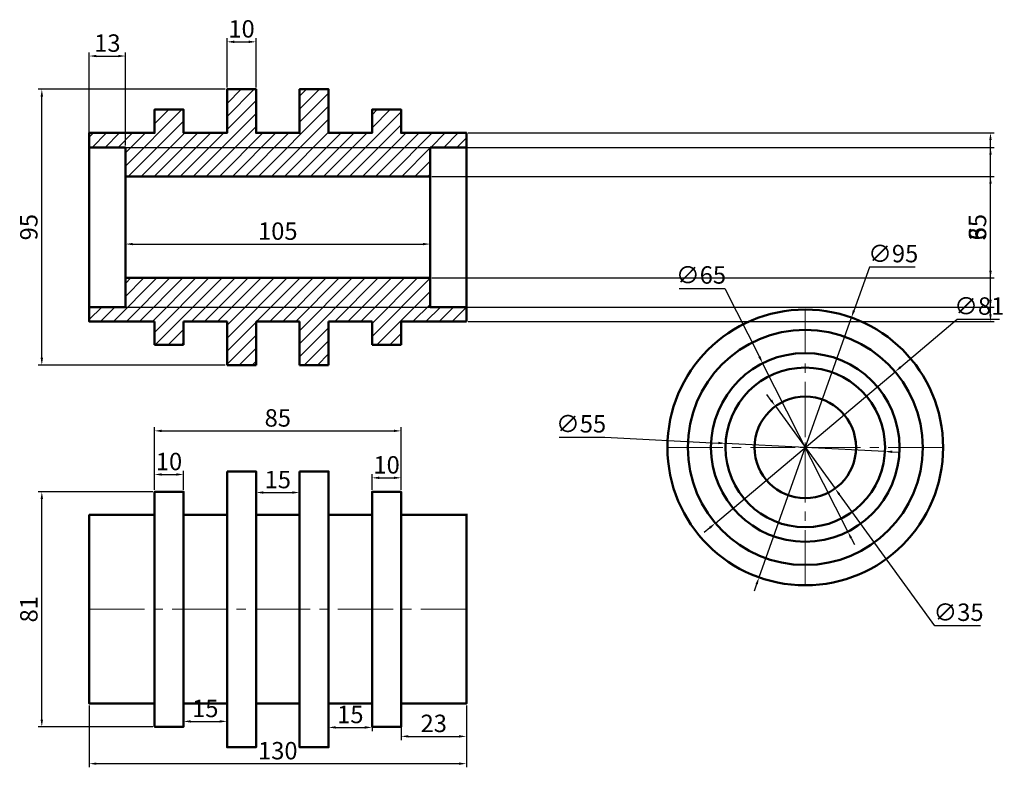
# Model space of a CAD drawing. Units: millimetres. Extents: x 106 to 445, y 110 to 368.
import ezdxf

# ---------------------------------------------------------------- set-up
doc = ezdxf.new("R2010")
doc.units = ezdxf.units.MM
doc.linetypes.add('CENTER2', pattern=[28.575, 19.05, -3.175, 3.175, -3.175])
for name, color, linetype, lineweight in [('M-CNTR', 4, 'CENTER2', 18), ('M-DIMS', 2, 'Continuous', 25), ('M-HATC', 8, 'Continuous', 18), ('M-OUTL', 7, 'Continuous', 50)]:
    doc.layers.add(name, color=color, linetype=linetype, lineweight=lineweight)
doc.styles.get("Standard").update_dxf_attribs({"font": 'arial.ttf'})
doc.dimstyles.new('ISO-25', dxfattribs={"dimtxt": 6, "dimasz": 2.5, "dimexe": 1.25, "dimexo": 0.625, "dimtad": 1, "dimtoh": 1, "dimdec": 0, "dimtxsty": 'Standard', "dimcen": 2.5, "dimadec": 0, "dimazin": 0, "dimtfac": 1, "dimtdec": 0, "dimtmove": 0, "dimatfit": 3, "dimfxl": 1, "dimarcsym": 0})

# ---------------------------------------------------------------- blocks, each defined once
blk = doc.blocks.new('*D1')
at = {"layer": 'Defpoints', "color": 0, "transparency": 16777216}
for p in [(142.24, 355.39), (129.74, 323.93), (142.24, 323.93)]:
    blk.add_point(p, dxfattribs=at)
at = {"layer": 'M-DIMS', "color": 0, "lineweight": -2, "transparency": 16777216}
for p, q in [((129.74, 324.56), (129.74, 356.64)), ((142.24, 324.56), (142.24, 356.64)), ((132.24, 355.39), (139.74, 355.39))]:
    blk.add_line(p, q, dxfattribs=at)
at = {"layer": 'M-DIMS', "color": 0, "transparency": 16777216}
for points in [[(132.24, 355.81), (132.24, 354.98), (129.74, 355.39)], [(139.74, 355.81), (139.74, 354.98), (142.24, 355.39)]]:
    blk.add_solid(points, dxfattribs=at)
at = {"layer": 'M-DIMS', "color": 0, "transparency": 16777216, "insert": (135.99, 359.08), "char_height": 6, "attachment_point": 5}
blk.add_mtext('13', dxfattribs=at)
blk = doc.blocks.new('*D2')
at = {"layer": 'Defpoints', "color": 0, "transparency": 16777216}
for p in [(142.24, 296.43), (247.24, 296.43), (247.24, 290.61)]:
    blk.add_point(p, dxfattribs=at)
at = {"layer": 'M-DIMS', "color": 0, "lineweight": -2, "transparency": 16777216}
for p, q in [((142.24, 295.81), (142.24, 289.36)), ((247.24, 295.81), (247.24, 289.36)), ((144.74, 290.61), (244.74, 290.61))]:
    blk.add_line(p, q, dxfattribs=at)
at = {"layer": 'M-DIMS', "color": 0, "transparency": 16777216}
for points in [[(144.74, 291.03), (144.74, 290.2), (142.24, 290.61)], [(244.74, 291.03), (244.74, 290.2), (247.24, 290.61)]]:
    blk.add_solid(points, dxfattribs=at)
at = {"layer": 'M-DIMS', "color": 0, "transparency": 16777216, "insert": (194.74, 294.3), "char_height": 6, "attachment_point": 5}
blk.add_mtext('105', dxfattribs=at)
blk = doc.blocks.new('*D3')
at = {"layer": 'Defpoints', "color": 0, "transparency": 16777216}
for p in [(237.24, 226.26), (152.24, 205.31), (237.24, 205.31)]:
    blk.add_point(p, dxfattribs=at)
at = {"layer": 'M-DIMS', "color": 0, "lineweight": -2, "transparency": 16777216}
for p, q in [((152.24, 205.93), (152.24, 227.51)), ((237.24, 205.93), (237.24, 227.51)), ((154.74, 226.26), (234.74, 226.26))]:
    blk.add_line(p, q, dxfattribs=at)
at = {"layer": 'M-DIMS', "color": 0, "transparency": 16777216}
for points in [[(154.74, 226.68), (154.74, 225.84), (152.24, 226.26)], [(234.74, 226.68), (234.74, 225.84), (237.24, 226.26)]]:
    blk.add_solid(points, dxfattribs=at)
at = {"layer": 'M-DIMS', "color": 0, "transparency": 16777216, "insert": (194.74, 229.95), "char_height": 6, "attachment_point": 5}
blk.add_mtext('85', dxfattribs=at)
blk = doc.blocks.new('*D4')
at = {"layer": 'Defpoints', "color": 0, "transparency": 16777216}
for p in [(129.74, 132.31), (259.74, 132.31), (259.74, 111.62)]:
    blk.add_point(p, dxfattribs=at)
at = {"layer": 'M-DIMS', "color": 0, "lineweight": -2, "transparency": 16777216}
for p, q in [((129.74, 131.68), (129.74, 110.37)), ((259.74, 131.68), (259.74, 110.37)), ((132.24, 111.62), (257.24, 111.62))]:
    blk.add_line(p, q, dxfattribs=at)
at = {"layer": 'M-DIMS', "color": 0, "transparency": 16777216}
for points in [[(132.24, 112.03), (132.24, 111.2), (129.74, 111.62)], [(257.24, 112.03), (257.24, 111.2), (259.74, 111.62)]]:
    blk.add_solid(points, dxfattribs=at)
at = {"layer": 'M-DIMS', "color": 0, "transparency": 16777216, "insert": (194.74, 115.31), "char_height": 6, "attachment_point": 5}
blk.add_mtext('130', dxfattribs=at)
blk = doc.blocks.new('*D5')
at = {"layer": 'Defpoints', "color": 0, "transparency": 16777216}
for p in [(162.24, 132.3), (177.24, 132.3), (177.24, 126.18)]:
    blk.add_point(p, dxfattribs=at)
at = {"layer": 'M-DIMS', "color": 0, "lineweight": -2, "transparency": 16777216}
for p, q in [((162.24, 131.67), (162.24, 124.93)), ((177.24, 131.67), (177.24, 124.93)), ((164.74, 126.18), (174.74, 126.18))]:
    blk.add_line(p, q, dxfattribs=at)
at = {"layer": 'M-DIMS', "color": 0, "transparency": 16777216}
for points in [[(164.74, 126.6), (164.74, 125.76), (162.24, 126.18)], [(174.74, 126.6), (174.74, 125.76), (177.24, 126.18)]]:
    blk.add_solid(points, dxfattribs=at)
at = {"layer": 'M-DIMS', "color": 0, "transparency": 16777216, "insert": (169.74, 129.87), "char_height": 6, "attachment_point": 5}
blk.add_mtext('15', dxfattribs=at)
blk = doc.blocks.new('*D6')
at = {"layer": 'Defpoints', "color": 0, "transparency": 16777216}
for p in [(162.24, 211.24), (152.24, 205.31), (162.24, 205.31)]:
    blk.add_point(p, dxfattribs=at)
at = {"layer": 'M-DIMS', "color": 0, "lineweight": -2, "transparency": 16777216}
for p, q in [((152.24, 205.93), (152.24, 212.49)), ((154.74, 211.24), (159.74, 211.24)), ((162.24, 205.93), (162.24, 212.49))]:
    blk.add_line(p, q, dxfattribs=at)
at = {"layer": 'M-DIMS', "color": 0, "transparency": 16777216}
for points in [[(154.74, 211.66), (154.74, 210.83), (152.24, 211.24)], [(159.74, 211.66), (159.74, 210.83), (162.24, 211.24)]]:
    blk.add_solid(points, dxfattribs=at)
at = {"layer": 'M-DIMS', "color": 0, "transparency": 16777216, "insert": (157.24, 214.93), "char_height": 6, "attachment_point": 5}
blk.add_mtext('10', dxfattribs=at)
blk = doc.blocks.new('*D7')
at = {"layer": 'Defpoints', "color": 0, "transparency": 16777216}
for p in [(237.24, 210.09), (227.24, 205.3), (237.24, 205.31)]:
    blk.add_point(p, dxfattribs=at)
at = {"layer": 'M-DIMS', "color": 0, "lineweight": -2, "transparency": 16777216}
for p, q in [((227.24, 205.92), (227.24, 211.34)), ((237.24, 205.93), (237.24, 211.34)), ((229.74, 210.09), (234.74, 210.09))]:
    blk.add_line(p, q, dxfattribs=at)
at = {"layer": 'M-DIMS', "color": 0, "transparency": 16777216}
for points in [[(229.74, 210.51), (229.74, 209.67), (227.24, 210.09)], [(234.74, 210.51), (234.74, 209.67), (237.24, 210.09)]]:
    blk.add_solid(points, dxfattribs=at)
at = {"layer": 'M-DIMS', "color": 0, "transparency": 16777216, "insert": (232.24, 213.78), "char_height": 6, "attachment_point": 5}
blk.add_mtext('10', dxfattribs=at)
blk = doc.blocks.new('*D8')
at = {"layer": 'Defpoints', "color": 0, "transparency": 16777216}
for p in [(202.24, 205.02), (187.24, 197.31), (202.24, 197.31)]:
    blk.add_point(p, dxfattribs=at)
at = {"layer": 'M-DIMS', "color": 0, "lineweight": -2, "transparency": 16777216}
for p, q in [((187.24, 197.93), (187.24, 206.27)), ((189.74, 205.02), (199.74, 205.02)), ((202.24, 197.93), (202.24, 206.27))]:
    blk.add_line(p, q, dxfattribs=at)
at = {"layer": 'M-DIMS', "color": 0, "transparency": 16777216}
for points in [[(189.74, 205.44), (189.74, 204.61), (187.24, 205.02)], [(199.74, 205.44), (199.74, 204.61), (202.24, 205.02)]]:
    blk.add_solid(points, dxfattribs=at)
at = {"layer": 'M-DIMS', "color": 0, "transparency": 16777216, "insert": (194.74, 208.71), "char_height": 6, "attachment_point": 5}
blk.add_mtext('15', dxfattribs=at)
blk = doc.blocks.new('*D9')
at = {"layer": 'Defpoints', "color": 0, "transparency": 16777216}
for p in [(212.24, 132.3), (227.24, 132.3), (227.24, 124.11)]:
    blk.add_point(p, dxfattribs=at)
at = {"layer": 'M-DIMS', "color": 0, "lineweight": -2, "transparency": 16777216}
for p, q in [((212.24, 131.67), (212.24, 122.86)), ((227.24, 131.67), (227.24, 122.86)), ((214.74, 124.11), (224.74, 124.11))]:
    blk.add_line(p, q, dxfattribs=at)
at = {"layer": 'M-DIMS', "color": 0, "transparency": 16777216}
for points in [[(214.74, 124.52), (214.74, 123.69), (212.24, 124.11)], [(224.74, 124.52), (224.74, 123.69), (227.24, 124.11)]]:
    blk.add_solid(points, dxfattribs=at)
at = {"layer": 'M-DIMS', "color": 0, "transparency": 16777216, "insert": (219.74, 127.79), "char_height": 6, "attachment_point": 5}
blk.add_mtext('15', dxfattribs=at)
blk = doc.blocks.new('*D10')
at = {"layer": 'Defpoints', "color": 0, "transparency": 16777216}
for p in [(237.24, 132.3), (259.74, 132.3), (259.74, 121.02)]:
    blk.add_point(p, dxfattribs=at)
at = {"layer": 'M-DIMS', "color": 0, "lineweight": -2, "transparency": 16777216}
for p, q in [((237.24, 131.67), (237.24, 119.77)), ((259.74, 131.67), (259.74, 119.77)), ((239.74, 121.02), (257.24, 121.02))]:
    blk.add_line(p, q, dxfattribs=at)
at = {"layer": 'M-DIMS', "color": 0, "transparency": 16777216}
for points in [[(239.74, 121.44), (239.74, 120.61), (237.24, 121.02)], [(257.24, 121.44), (257.24, 120.61), (259.74, 121.02)]]:
    blk.add_solid(points, dxfattribs=at)
at = {"layer": 'M-DIMS', "color": 0, "transparency": 16777216, "insert": (248.49, 124.72), "char_height": 6, "attachment_point": 5}
blk.add_mtext('23', dxfattribs=at)
blk = doc.blocks.new('*D11')
at = {"layer": 'Defpoints', "color": 0, "transparency": 16777216}
for p in [(366.27, 234.72), (386.85, 206.41)]:
    blk.add_point(p, dxfattribs=at)
at = {"layer": 'M-DIMS', "color": 0, "lineweight": -2, "transparency": 16777216}
for p, q in [((364.8, 236.74), (363.33, 238.76)), ((366.27, 234.72), (386.85, 206.41)), ((421.18, 159.15), (388.32, 204.38)), ((436.98, 159.15), (421.18, 159.15))]:
    blk.add_line(p, q, dxfattribs=at)
at = {"layer": 'M-DIMS', "color": 0, "transparency": 16777216}
for points in [[(365.14, 236.99), (364.47, 236.5), (366.27, 234.72)], [(388.65, 204.63), (387.98, 204.14), (386.85, 206.41)]]:
    blk.add_solid(points, dxfattribs=at)
at = {"layer": 'M-DIMS', "color": 0, "transparency": 16777216, "insert": (429.39, 163.01), "char_height": 6, "attachment_point": 5}
blk.add_mtext('∅35', dxfattribs=at)
blk = doc.blocks.new('*D12')
at = {"layer": 'Defpoints', "color": 0, "transparency": 16777216}
for p in [(349.1, 221.96), (404.02, 219.17)]:
    blk.add_point(p, dxfattribs=at)
at = {"layer": 'M-DIMS', "color": 0, "lineweight": -2, "transparency": 16777216}
for p, q in [((291.71, 224.06), (307.5, 224.06)), ((307.5, 224.06), (346.6, 222.08)), ((404.02, 219.17), (349.1, 221.96)), ((406.52, 219.04), (409.02, 218.92))]:
    blk.add_line(p, q, dxfattribs=at)
at = {"layer": 'M-DIMS', "color": 0, "transparency": 16777216}
for points in [[(346.62, 222.5), (346.58, 221.67), (349.1, 221.96)], [(406.54, 219.46), (406.5, 218.63), (404.02, 219.17)]]:
    blk.add_solid(points, dxfattribs=at)
at = {"layer": 'M-DIMS', "color": 0, "transparency": 16777216, "insert": (299.29, 227.92), "char_height": 6, "attachment_point": 5}
blk.add_mtext('∅55', dxfattribs=at)
blk = doc.blocks.new('*D13')
at = {"layer": 'Defpoints', "color": 0, "transparency": 16777216}
for p in [(361.88, 249.56), (391.24, 191.57)]:
    blk.add_point(p, dxfattribs=at)
at = {"layer": 'M-DIMS', "color": 0, "lineweight": -2, "transparency": 16777216}
for p, q in [((333.05, 275.33), (348.84, 275.33)), ((348.84, 275.33), (360.75, 251.79)), ((391.24, 191.57), (361.88, 249.56)), ((392.37, 189.33), (393.5, 187.1))]:
    blk.add_line(p, q, dxfattribs=at)
at = {"layer": 'M-DIMS', "color": 0, "transparency": 16777216}
for points in [[(361.13, 251.98), (360.38, 251.6), (361.88, 249.56)], [(392.74, 189.52), (391.99, 189.15), (391.24, 191.57)]]:
    blk.add_solid(points, dxfattribs=at)
at = {"layer": 'M-DIMS', "color": 0, "transparency": 16777216, "insert": (340.63, 279.19), "char_height": 6, "attachment_point": 5}
blk.add_mtext('∅65', dxfattribs=at)
blk = doc.blocks.new('*D14')
at = {"layer": 'Defpoints', "color": 0, "transparency": 16777216}
for p in [(407.55, 246.64), (345.57, 194.49)]:
    blk.add_point(p, dxfattribs=at)
at = {"layer": 'M-DIMS', "color": 0, "lineweight": -2, "transparency": 16777216}
for p, q in [((428.93, 264.63), (409.46, 248.25)), ((443.52, 264.63), (428.93, 264.63)), ((345.57, 194.49), (407.55, 246.64)), ((343.66, 192.88), (341.75, 191.27))]:
    blk.add_line(p, q, dxfattribs=at)
at = {"layer": 'M-DIMS', "color": 0, "transparency": 16777216}
for points in [[(409.19, 248.57), (409.73, 247.93), (407.55, 246.64)], [(343.39, 193.2), (343.93, 192.56), (345.57, 194.49)]]:
    blk.add_solid(points, dxfattribs=at)
at = {"layer": 'M-DIMS', "color": 0, "transparency": 16777216, "insert": (436.54, 268.49), "char_height": 6, "attachment_point": 5}
blk.add_mtext('∅81', dxfattribs=at)
blk = doc.blocks.new('*D15')
at = {"layer": 'Defpoints', "color": 0, "transparency": 16777216}
for p in [(392.48, 265.31), (360.64, 175.81)]:
    blk.add_point(p, dxfattribs=at)
at = {"layer": 'M-DIMS', "color": 0, "lineweight": -2, "transparency": 16777216}
for p, q in [((398.67, 282.71), (393.32, 267.67)), ((414.46, 282.71), (398.67, 282.71)), ((360.64, 175.81), (392.48, 265.31)), ((359.8, 173.45), (358.96, 171.1))]:
    blk.add_line(p, q, dxfattribs=at)
at = {"layer": 'M-DIMS', "color": 0, "transparency": 16777216}
for points in [[(392.93, 267.81), (393.71, 267.53), (392.48, 265.31)], [(359.41, 173.59), (360.19, 173.32), (360.64, 175.81)]]:
    blk.add_solid(points, dxfattribs=at)
at = {"layer": 'M-DIMS', "color": 0, "transparency": 16777216, "insert": (406.88, 286.56), "char_height": 6, "attachment_point": 5}
blk.add_mtext('∅95', dxfattribs=at)
blk = doc.blocks.new('*D16')
at = {"layer": 'Defpoints', "color": 0, "transparency": 16777216}
for p in [(113.39, 343.93), (177.24, 343.93), (177.24, 248.93)]:
    blk.add_point(p, dxfattribs=at)
at = {"layer": 'M-DIMS', "color": 0, "lineweight": -2, "transparency": 16777216}
for p, q in [((176.62, 343.93), (112.14, 343.93)), ((113.39, 251.43), (113.39, 341.43)), ((176.62, 248.93), (112.14, 248.93))]:
    blk.add_line(p, q, dxfattribs=at)
at = {"layer": 'M-DIMS', "color": 0, "transparency": 16777216}
for points in [[(112.98, 341.43), (113.81, 341.43), (113.39, 343.93)], [(112.98, 251.43), (113.81, 251.43), (113.39, 248.93)]]:
    blk.add_solid(points, dxfattribs=at)
at = {"layer": 'M-DIMS', "color": 0, "transparency": 16777216, "insert": (109.7, 296.43), "char_height": 6, "attachment_point": 5, "rotation": 90}
blk.add_mtext('95', dxfattribs=at)
blk = doc.blocks.new('*D17')
at = {"layer": 'Defpoints', "color": 0, "transparency": 16777216}
for p in [(259.74, 328.93), (440.41, 328.93), (259.74, 263.93)]:
    blk.add_point(p, dxfattribs=at)
at = {"layer": 'M-DIMS', "color": 0, "lineweight": -2, "transparency": 16777216}
for p, q in [((260.37, 328.93), (441.66, 328.93)), ((440.41, 266.43), (440.41, 326.43)), ((260.37, 263.93), (441.66, 263.93))]:
    blk.add_line(p, q, dxfattribs=at)
at = {"layer": 'M-DIMS', "color": 0, "transparency": 16777216}
for points in [[(439.99, 326.43), (440.83, 326.43), (440.41, 328.93)], [(439.99, 266.43), (440.83, 266.43), (440.41, 263.93)]]:
    blk.add_solid(points, dxfattribs=at)
at = {"layer": 'M-DIMS', "color": 0, "transparency": 16777216, "insert": (436.72, 296.43), "char_height": 6, "attachment_point": 5, "rotation": 90}
blk.add_mtext('65', dxfattribs=at)
blk = doc.blocks.new('*D18')
at = {"layer": 'Defpoints', "color": 0, "transparency": 16777216}
for p in [(113.39, 205.31), (152.24, 205.31), (152.24, 124.31)]:
    blk.add_point(p, dxfattribs=at)
at = {"layer": 'M-DIMS', "color": 0, "lineweight": -2, "transparency": 16777216}
for p, q in [((151.62, 205.31), (112.14, 205.31)), ((113.39, 126.81), (113.39, 202.81)), ((151.62, 124.31), (112.14, 124.31))]:
    blk.add_line(p, q, dxfattribs=at)
at = {"layer": 'M-DIMS', "color": 0, "transparency": 16777216}
for points in [[(112.98, 202.81), (113.81, 202.81), (113.39, 205.31)], [(112.98, 126.81), (113.81, 126.81), (113.39, 124.31)]]:
    blk.add_solid(points, dxfattribs=at)
at = {"layer": 'M-DIMS', "color": 0, "transparency": 16777216, "insert": (109.7, 164.81), "char_height": 6, "attachment_point": 5, "rotation": 90}
blk.add_mtext('81', dxfattribs=at)
blk = doc.blocks.new('*D19')
at = {"layer": 'Defpoints', "color": 0, "transparency": 16777216}
for p in [(129.74, 323.93), (440.41, 323.93), (129.74, 268.93)]:
    blk.add_point(p, dxfattribs=at)
at = {"layer": 'M-DIMS', "color": 0, "lineweight": -2, "transparency": 16777216}
for p, q in [((130.37, 323.93), (441.66, 323.93)), ((440.41, 271.43), (440.41, 321.43)), ((130.37, 268.93), (441.66, 268.93))]:
    blk.add_line(p, q, dxfattribs=at)
at = {"layer": 'M-DIMS', "color": 0, "transparency": 16777216}
for points in [[(439.99, 321.43), (440.83, 321.43), (440.41, 323.93)], [(439.99, 271.43), (440.83, 271.43), (440.41, 268.93)]]:
    blk.add_solid(points, dxfattribs=at)
at = {"layer": 'M-DIMS', "color": 0, "transparency": 16777216, "insert": (436.73, 296.43), "char_height": 6, "attachment_point": 5, "rotation": 90}
blk.add_mtext('55', dxfattribs=at)
blk = doc.blocks.new('*D20')
at = {"layer": 'Defpoints', "color": 0, "transparency": 16777216}
for p in [(247.24, 313.93), (440.41, 313.93), (247.24, 278.93)]:
    blk.add_point(p, dxfattribs=at)
at = {"layer": 'M-DIMS', "color": 0, "lineweight": -2, "transparency": 16777216}
for p, q in [((247.87, 313.93), (441.66, 313.93)), ((440.41, 281.43), (440.41, 311.43)), ((247.87, 278.93), (441.66, 278.93))]:
    blk.add_line(p, q, dxfattribs=at)
at = {"layer": 'M-DIMS', "color": 0, "transparency": 16777216}
for points in [[(439.99, 311.43), (440.83, 311.43), (440.41, 313.93)], [(439.99, 281.43), (440.83, 281.43), (440.41, 278.93)]]:
    blk.add_solid(points, dxfattribs=at)
at = {"layer": 'M-DIMS', "color": 0, "transparency": 16777216, "insert": (436.72, 296.43), "char_height": 6, "attachment_point": 5, "rotation": 90}
blk.add_mtext('35', dxfattribs=at)
blk = doc.blocks.new('*D21')
at = {"layer": 'Defpoints', "color": 0, "transparency": 16777216}
for p in [(187.24, 360.28), (177.24, 343.93), (187.24, 343.93)]:
    blk.add_point(p, dxfattribs=at)
at = {"layer": 'M-DIMS', "color": 0, "lineweight": -2, "transparency": 16777216}
for p, q in [((177.24, 344.56), (177.24, 361.53)), ((179.74, 360.28), (184.74, 360.28)), ((187.24, 344.56), (187.24, 361.53))]:
    blk.add_line(p, q, dxfattribs=at)
at = {"layer": 'M-DIMS', "color": 0, "transparency": 16777216}
for points in [[(179.74, 360.7), (179.74, 359.87), (177.24, 360.28)], [(184.74, 360.7), (184.74, 359.87), (187.24, 360.28)]]:
    blk.add_solid(points, dxfattribs=at)
at = {"layer": 'M-DIMS', "color": 0, "transparency": 16777216, "insert": (182.24, 363.97), "char_height": 6, "attachment_point": 5}
blk.add_mtext('10', dxfattribs=at)

msp = doc.modelspace()

# ---------------------------------------------------------------- hatches: boundary and pattern name
at = {"layer": 'M-HATC'}
h = msp.add_hatch(dxfattribs=at)
h.set_pattern_fill('ANSI31', color=256)
h.set_pattern_definition([(45, (101.0912, 253.9006), (-2.245064, 2.245064), [])])
h.paths.add_polyline_path([(152.24, 328.93), (142.24, 328.93), (129.74, 328.93), (129.74, 323.93), (142.24, 323.93), (142.24, 313.93), (247.24, 313.93), (247.24, 323.93), (259.74, 323.93), (259.74, 328.93), (237.24, 328.93), (237.24, 336.93), (227.24, 336.93), (227.24, 328.93), (212.24, 328.93), (212.24, 343.93), (202.24, 343.93), (202.24, 328.93), (187.24, 328.93), (187.24, 343.93), (177.24, 343.93), (177.24, 328.93), (162.24, 328.93), (162.24, 336.93), (152.24, 336.93)])
h.paths.add_polyline_path([(142.24, 278.93), (142.24, 268.93), (129.74, 268.93), (129.74, 266.43), (129.74, 263.93), (142.24, 263.93), (152.24, 263.93), (152.24, 255.93), (162.24, 255.93), (162.24, 263.93), (177.24, 263.93), (177.24, 248.93), (187.24, 248.93), (187.24, 263.93), (202.24, 263.93), (202.24, 248.93), (212.24, 248.93), (212.24, 263.93), (227.24, 263.93), (227.24, 255.93), (237.24, 255.93), (237.24, 263.93), (259.74, 263.93), (259.74, 268.93), (247.24, 268.93), (247.24, 278.93)])

# ---------------------------------------------------------------- linework, layer by layer
at = {"layer": 'M-CNTR'}
for p, q in [((376.56, 224.06), (376.56, 268.06)), ((376.56, 218.81), (376.56, 222.31)), ((329.06, 220.56), (373.06, 220.56)), ((374.81, 220.56), (378.31, 220.56)), ((129.74, 164.81), (259.74, 164.81))]:
    msp.add_line(p, q, dxfattribs=at)
msp.add_lwpolyline([(376.56, 173.06), (376.56, 220.56), (424.06, 220.56)], dxfattribs=at)
at = {"layer": 'M-OUTL'}
for p, q in [((142.24, 313.93), (247.24, 313.93)), ((142.24, 278.93), (247.24, 278.93)), ((259.74, 268.93), (259.74, 263.93)), ((142.24, 263.93), (152.24, 263.93)), ((142.24, 263.93), (152.24, 263.93)), ((152.24, 263.93), (152.24, 255.93)), ((162.24, 255.93), (162.24, 263.93)), ((162.24, 263.93), (177.24, 263.93)), ((177.24, 263.93), (177.24, 248.93)), ((187.24, 248.93), (187.24, 263.93)), ((187.24, 263.93), (202.24, 263.93)), ((202.24, 263.93), (202.24, 248.93)), ((212.24, 248.93), (212.24, 263.93)), ((212.24, 263.93), (227.24, 263.93)), ((227.24, 263.93), (227.24, 255.93)), ((259.74, 263.93), (237.24, 263.93)), ((237.24, 255.93), (237.24, 263.93)), ((152.24, 255.93), (162.24, 255.93)), ((227.24, 255.93), (237.24, 255.93)), ((177.24, 248.93), (187.24, 248.93)), ((202.24, 248.93), (212.24, 248.93)), ((162.24, 197.31), (177.24, 197.31)), ((187.24, 197.31), (202.24, 197.31)), ((212.24, 197.31), (227.24, 197.31)), ((237.24, 197.31), (259.74, 197.31)), ((162.24, 132.3), (177.24, 132.3)), ((187.24, 132.3), (202.24, 132.3)), ((212.24, 132.3), (227.24, 132.3))]:
    msp.add_line(p, q, dxfattribs=at)
for points in [[(129.74, 323.93), (129.74, 328.93), (142.24, 328.93), (152.24, 328.93), (152.24, 336.93), (162.24, 336.93), (162.24, 328.93), (177.24, 328.93), (177.24, 343.93), (187.24, 343.93), (187.24, 328.93), (202.24, 328.93), (202.24, 343.93), (212.24, 343.93), (212.24, 328.93), (227.24, 328.93), (227.24, 336.93), (237.24, 336.93), (237.24, 328.93), (259.74, 328.93), (259.74, 323.93)], [(142.24, 263.93), (129.74, 263.93), (129.74, 268.93), (142.24, 268.93), (142.24, 323.93), (129.74, 323.93), (129.74, 266.43)], [(152.24, 197.31), (129.74, 197.31), (129.74, 132.31), (152.24, 132.31)], [(237.24, 132.3), (259.74, 132.3), (259.74, 197.74)]]:
    msp.add_lwpolyline(points, dxfattribs=at)
for points in [[(247.24, 323.93), (247.24, 268.93), (259.74, 268.93), (259.74, 323.93)], [(177.24, 212.31), (187.24, 212.31), (187.24, 117.3), (177.24, 117.3), (177.24, 197.56)], [(202.24, 212.31), (212.24, 212.31), (212.24, 117.3), (202.24, 117.3), (202.24, 197.74)], [(152.24, 197.31), (152.24, 205.31), (162.24, 205.31), (162.24, 124.31), (152.24, 124.31), (152.24, 132.31), (152.24, 164.81)], [(227.24, 124.3), (237.24, 124.3), (237.24, 205.3), (227.24, 205.3), (227.24, 197.74), (227.24, 132.3)]]:
    msp.add_lwpolyline(points, close=True, dxfattribs=at)
for radius in [47.5, 40.5, 32.5, 27.5, 17.5]:
    msp.add_circle((376.56, 220.56), radius, dxfattribs=at)

# ---------------------------------------------------------------- dimensions: what is measured, and where the dimension line sits
at = {"layer": 'M-DIMS'}
for base, p1, p2, override, picture, middle in [((187.24, 360.28), (177.24, 343.93), (187.24, 343.93), {"dimdec": 0, "dimlfac": 1, "dimrnd": 0, "dimzin": 0, "dimdsep": 46, "dimlunit": 2}, '*D21', (182.24, 363.97)), ((142.24278027, 355.39239272), (129.74278027, 323.93260068), (142.24278027, 323.93260068), {"dimclrd": 0, "dimclre": 0, "dimclrt": 0}, '*D1', (135.99278027, 359.08287703)), ((247.24, 290.61), (142.24, 296.43), (247.24, 296.43), {"dimclrd": 0, "dimclre": 0, "dimclrt": 0}, '*D2', (194.74, 294.3)), ((237.24, 226.26), (152.24, 205.31), (237.24, 205.31), {"dimclrd": 0, "dimclre": 0, "dimclrt": 0}, '*D3', (194.74, 229.95)), ((162.24, 211.24), (152.24, 205.31), (162.24, 205.31), {"dimclrd": 0, "dimclre": 0, "dimclrt": 0}, '*D6', (157.24, 214.93)), ((237.24, 210.09), (227.24, 205.3), (237.24, 205.31), {"dimclrd": 0, "dimclre": 0, "dimclrt": 0}, '*D7', (232.24, 213.78)), ((202.24, 205.02), (187.24, 197.31), (202.24, 197.31), {"dimclrd": 0, "dimclre": 0, "dimclrt": 0}, '*D8', (194.74, 208.71)), ((177.24, 126.18), (162.24, 132.3), (177.24, 132.3), {"dimclrd": 0, "dimclre": 0, "dimclrt": 0}, '*D5', (169.74, 129.87)), ((259.74, 111.62), (129.74, 132.31), (259.74, 132.31), {"dimclrd": 0, "dimclre": 0, "dimclrt": 0}, '*D4', (194.74, 115.31)), ((227.24, 124.11), (212.24, 132.3), (227.24, 132.3), {"dimclrd": 0, "dimclre": 0, "dimclrt": 0}, '*D9', (219.74, 127.79)), ((259.74278027, 121.02497396), (237.24278027, 132.29816493), (259.74278027, 132.29816493), {"dimclrd": 0, "dimclre": 0, "dimclrt": 0}, '*D10', (248.49278027, 124.71545827))]:
    dim = msp.add_linear_dim(base=base, p1=p1, p2=p2, dimstyle='ISO-25', override=override, dxfattribs=at)
    dim.commit()
    dim.dimension.update_dxf_attribs({"geometry": picture, "text_midpoint": middle})
for base, p1, p2, picture, middle in [((113.39, 343.93), (177.24, 248.93), (177.24, 343.93), '*D16', (109.7, 296.43)), ((440.41, 328.93), (259.74, 263.93), (259.74, 328.93), '*D17', (436.72, 296.43)), ((440.41, 323.93), (129.74, 268.93), (129.74, 323.93), '*D19', (436.73, 296.43)), ((440.41, 313.93), (247.24, 278.93), (247.24, 313.93), '*D20', (436.72, 296.43)), ((113.39, 205.31), (152.24, 124.31), (152.24, 205.31), '*D18', (109.7, 164.81))]:
    dim = msp.add_linear_dim(base=base, p1=p1, p2=p2, angle=90, dimstyle='ISO-25', override={"dimdec": 0, "dimlfac": 1, "dimrnd": 0, "dimzin": 0, "dimdsep": 46, "dimlunit": 2}, dxfattribs=at)
    dim.commit()
    dim.dimension.update_dxf_attribs({"geometry": picture, "text_midpoint": middle})
for p1, p2, picture, middle in [((360.64, 175.81), (392.48, 265.31), '*D15', (406.88, 282.71)), ((391.24, 191.57), (361.88, 249.56), '*D13', (340.63, 275.33)), ((345.57, 194.49), (407.55, 246.64), '*D14', (436.54, 264.63)), ((366.27, 234.72), (386.85, 206.41), '*D11', (429.39, 159.15)), ((404.02, 219.17), (349.1, 221.96), '*D12', (307.5, 224.06))]:
    dim = msp.add_diameter_dim_2p(p1=p1, p2=p2, dimstyle='ISO-25', override={"dimclrd": 0, "dimclre": 0, "dimclrt": 0}, dxfattribs=at)
    dim.commit()
    dim.dimension.update_dxf_attribs({"geometry": picture, "text_midpoint": middle, "dimtype": 163})

doc.saveas('drawing.dxf')
